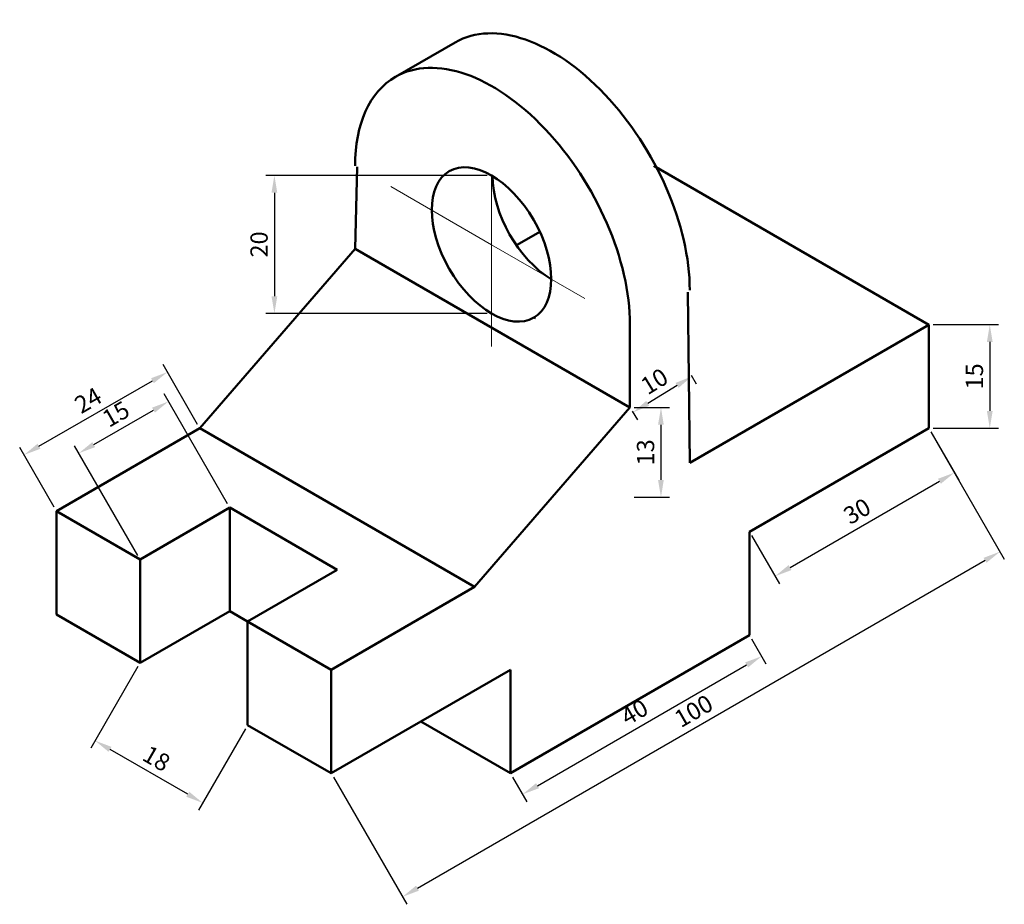
# Model space of a CAD drawing. Units: millimetres. Extents: x 20220 to 20363, y 7548 to 7676.
import ezdxf

# ---------------------------------------------------------------- set-up
doc = ezdxf.new("R2010")
doc.units = ezdxf.units.MM
doc.linetypes.add('CENTER', pattern=[50.8, 31.75, -6.35, 6.35, -6.35])
for name, color, linetype, lineweight in [('M-CNTR', 1, 'CENTER', 18), ('M-DIMS', 2, 'Continuous', 25), ('M-OUTL', 7, 'Continuous', 50)]:
    doc.layers.add(name, color=color, linetype=linetype, lineweight=lineweight)
doc.styles.get("Standard").update_dxf_attribs({"font": 'arial.ttf'})
doc.dimstyles.new('ISO-25', dxfattribs={"dimtxt": 2.5, "dimasz": 2.5, "dimexe": 1.25, "dimexo": 0.625, "dimtad": 1, "dimtxsty": 'Standard', "dimcen": 2.5, "dimadec": 0, "dimazin": 0, "dimtfac": 1, "dimtmove": 0, "dimatfit": 3, "dimfxl": 1, "dimarcsym": 0})

# ---------------------------------------------------------------- blocks, each defined once
blk = doc.blocks.new('*D1')
at = {"layer": 'Defpoints', "color": 0, "transparency": 16777216}
for p in [(20241.42, 7620.43), (20250.3, 7605.06), (20237.31, 7597.56)]:
    blk.add_point(p, dxfattribs=at)
at = {"layer": 'M-DIMS', "color": 0, "lineweight": -2, "transparency": 16777216}
for p, q in [((20249.98, 7605.6), (20240.79, 7621.52)), ((20230.59, 7614.18), (20239.25, 7619.18)), ((20236.99, 7598.1), (20227.8, 7614.02))]:
    blk.add_line(p, q, dxfattribs=at)
at = {"layer": 'M-DIMS', "color": 0, "transparency": 16777216}
for points in [[(20239.05, 7619.54), (20239.46, 7618.82), (20241.42, 7620.43)], [(20230.39, 7614.54), (20230.8, 7613.82), (20228.43, 7612.93)]]:
    blk.add_solid(points, dxfattribs=at)
at = {"layer": 'M-DIMS', "color": 0, "transparency": 16777216, "insert": (20233.97, 7618.33), "char_height": 2.5, "attachment_point": 5, "rotation": 30}
blk.add_mtext('15', dxfattribs=at)
blk = doc.blocks.new('*D2')
at = {"layer": 'Defpoints', "color": 0, "transparency": 16777216}
for p in [(20241.27, 7624.69), (20245.97, 7616.56), (20225.18, 7604.56)]:
    blk.add_point(p, dxfattribs=at)
at = {"layer": 'M-DIMS', "color": 0, "lineweight": -2, "transparency": 16777216}
for p, q in [((20245.65, 7617.1), (20240.65, 7625.77)), ((20222.65, 7613.94), (20239.11, 7623.44)), ((20224.87, 7605.1), (20219.86, 7613.77))]:
    blk.add_line(p, q, dxfattribs=at)
at = {"layer": 'M-DIMS', "color": 0, "transparency": 16777216}
for points in [[(20238.9, 7623.8), (20239.31, 7623.08), (20241.27, 7624.69)], [(20222.44, 7614.3), (20222.86, 7613.58), (20220.49, 7612.69)]]:
    blk.add_solid(points, dxfattribs=at)
at = {"layer": 'M-DIMS', "color": 0, "transparency": 16777216, "insert": (20229.94, 7620.32), "char_height": 2.5, "attachment_point": 5, "rotation": 30}
blk.add_mtext('24', dxfattribs=at)
blk = doc.blocks.new('*D3')
at = {"layer": 'Defpoints', "color": 0, "transparency": 16777216}
for p in [(20351.62, 7616.56), (20361.95, 7598.67), (20265.02, 7566.56)]:
    blk.add_point(p, dxfattribs=at)
at = {"layer": 'M-DIMS', "color": 0, "lineweight": -2, "transparency": 16777216}
for p, q in [((20351.93, 7616.02), (20362.58, 7597.58)), ((20277.51, 7549.92), (20359.79, 7597.42)), ((20265.33, 7566.02), (20275.97, 7547.58))]:
    blk.add_line(p, q, dxfattribs=at)
at = {"layer": 'M-DIMS', "color": 0, "transparency": 16777216}
for points in [[(20359.58, 7597.78), (20359.99, 7597.06), (20361.95, 7598.67)], [(20277.31, 7550.28), (20277.72, 7549.56), (20275.35, 7548.67)]]:
    blk.add_solid(points, dxfattribs=at)
at = {"layer": 'M-DIMS', "color": 0, "transparency": 16777216, "insert": (20317.7, 7575.31), "char_height": 2.5, "attachment_point": 5, "rotation": 30}
blk.add_mtext('100', dxfattribs=at)
blk = doc.blocks.new('*D4')
at = {"layer": 'Defpoints', "color": 0, "transparency": 16777216}
for p in [(20325.64, 7586.56), (20327.4, 7583.52), (20291, 7566.56)]:
    blk.add_point(p, dxfattribs=at)
at = {"layer": 'M-DIMS', "color": 0, "lineweight": -2, "transparency": 16777216}
for p, q in [((20325.95, 7586.02), (20328.02, 7582.43)), ((20294.92, 7564.77), (20325.23, 7582.27)), ((20291.31, 7566.02), (20293.38, 7562.43))]:
    blk.add_line(p, q, dxfattribs=at)
at = {"layer": 'M-DIMS', "color": 0, "transparency": 16777216}
for points in [[(20325.02, 7582.63), (20325.44, 7581.9), (20327.4, 7583.52)], [(20294.71, 7565.13), (20295.13, 7564.4), (20292.76, 7563.52)]]:
    blk.add_solid(points, dxfattribs=at)
at = {"layer": 'M-DIMS', "color": 0, "transparency": 16777216, "insert": (20309.13, 7575.16), "char_height": 2.5, "attachment_point": 5, "rotation": 30}
blk.add_mtext('40', dxfattribs=at)
blk = doc.blocks.new('*D5')
at = {"layer": 'Defpoints', "color": 0, "transparency": 16777216}
for p in [(20351.62, 7616.56), (20355.34, 7610.12), (20325.64, 7601.56)]:
    blk.add_point(p, dxfattribs=at)
at = {"layer": 'M-DIMS', "color": 0, "lineweight": -2, "transparency": 16777216}
for p, q in [((20351.93, 7616.02), (20355.97, 7609.03)), ((20331.52, 7596.37), (20353.18, 7608.87)), ((20325.95, 7601.02), (20329.98, 7594.03))]:
    blk.add_line(p, q, dxfattribs=at)
at = {"layer": 'M-DIMS', "color": 0, "transparency": 16777216}
for points in [[(20352.97, 7609.23), (20353.38, 7608.51), (20355.34, 7610.12)], [(20331.32, 7596.73), (20331.73, 7596.01), (20329.36, 7595.12)]]:
    blk.add_solid(points, dxfattribs=at)
at = {"layer": 'M-DIMS', "color": 0, "transparency": 16777216, "insert": (20341.4, 7604.26), "char_height": 2.5, "attachment_point": 5, "rotation": 30}
blk.add_mtext('30', dxfattribs=at)
blk = doc.blocks.new('*D6')
at = {"layer": 'Defpoints', "color": 0, "transparency": 16777216}
for p in [(20351.62, 7631.56), (20351.62, 7616.56), (20360.47, 7616.56)]:
    blk.add_point(p, dxfattribs=at)
at = {"layer": 'M-DIMS', "color": 0, "lineweight": -2, "transparency": 16777216}
for p, q in [((20352.25, 7631.56), (20361.72, 7631.56)), ((20360.47, 7629.06), (20360.47, 7619.06)), ((20352.25, 7616.56), (20361.72, 7616.56))]:
    blk.add_line(p, q, dxfattribs=at)
at = {"layer": 'M-DIMS', "color": 0, "transparency": 16777216}
for points in [[(20360.05, 7629.06), (20360.89, 7629.06), (20360.47, 7631.56)], [(20360.05, 7619.06), (20360.89, 7619.06), (20360.47, 7616.56)]]:
    blk.add_solid(points, dxfattribs=at)
at = {"layer": 'M-DIMS', "color": 0, "transparency": 16777216, "insert": (20358.57, 7624.06), "char_height": 2.5, "attachment_point": 5, "rotation": 90}
blk.add_mtext('15', dxfattribs=at)
blk = doc.blocks.new('*D7')
at = {"layer": 'Defpoints', "color": 0, "transparency": 16777216}
for p in [(20237.31, 7582.56), (20252.89, 7573.56), (20230.8, 7571.28)]:
    blk.add_point(p, dxfattribs=at)
at = {"layer": 'M-DIMS', "color": 0, "lineweight": -2, "transparency": 16777216}
for p, q in [((20236.99, 7582.02), (20230.17, 7570.2)), ((20252.58, 7573.02), (20245.76, 7561.2)), ((20244.22, 7563.53), (20232.96, 7570.03))]:
    blk.add_line(p, q, dxfattribs=at)
at = {"layer": 'M-DIMS', "color": 0, "transparency": 16777216}
for points in [[(20233.17, 7570.39), (20232.75, 7569.67), (20230.8, 7571.28)], [(20244.43, 7563.89), (20244.01, 7563.17), (20246.38, 7562.28)]]:
    blk.add_solid(points, dxfattribs=at)
at = {"layer": 'M-DIMS', "color": 0, "transparency": 16777216, "insert": (20239.54, 7568.43), "char_height": 2.5, "attachment_point": 5, "rotation": 330}
blk.add_mtext('18', dxfattribs=at)
blk = doc.blocks.new('*D8')
at = {"layer": 'Defpoints', "color": 0, "transparency": 16777216}
for p in [(20308.32, 7619.56), (20308.32, 7606.56), (20312.81, 7606.56)]:
    blk.add_point(p, dxfattribs=at)
at = {"layer": 'M-DIMS', "color": 0, "lineweight": -2, "transparency": 16777216}
for p, q in [((20308.95, 7619.56), (20314.06, 7619.56)), ((20312.81, 7617.06), (20312.81, 7609.06)), ((20308.95, 7606.56), (20314.06, 7606.56))]:
    blk.add_line(p, q, dxfattribs=at)
at = {"layer": 'M-DIMS', "color": 0, "transparency": 16777216}
for points in [[(20312.39, 7617.06), (20313.22, 7617.06), (20312.81, 7619.56)], [(20312.39, 7609.06), (20313.22, 7609.06), (20312.81, 7606.56)]]:
    blk.add_solid(points, dxfattribs=at)
at = {"layer": 'M-DIMS', "color": 0, "transparency": 16777216, "insert": (20310.9, 7613.06), "char_height": 2.5, "attachment_point": 5, "rotation": 90}
blk.add_mtext('13', dxfattribs=at)
blk = doc.blocks.new('*D9')
at = {"layer": 'Defpoints', "color": 0, "transparency": 16777216}
for p in [(20316.85, 7624.78), (20308.32, 7619.56), (20308.75, 7618.85)]:
    blk.add_point(p, dxfattribs=at)
at = {"layer": 'M-DIMS', "color": 0, "lineweight": -2, "transparency": 16777216}
for p, q in [((20317.18, 7624.25), (20317.93, 7623.01)), ((20315.15, 7622.77), (20310.89, 7620.16)), ((20308.65, 7619.03), (20309.41, 7617.79))]:
    blk.add_line(p, q, dxfattribs=at)
at = {"layer": 'M-DIMS', "color": 0, "transparency": 16777216}
for points in [[(20314.93, 7623.12), (20315.37, 7622.41), (20317.28, 7624.07)], [(20310.67, 7620.51), (20311.1, 7619.8), (20308.75, 7618.85)]]:
    blk.add_solid(points, dxfattribs=at)
at = {"layer": 'M-DIMS', "color": 0, "transparency": 16777216, "insert": (20312.02, 7623.08), "char_height": 2.5, "attachment_point": 5, "rotation": 31.4807}
blk.add_mtext('10', dxfattribs=at)
blk = doc.blocks.new('*D10')
at = {"layer": 'Defpoints', "color": 0, "transparency": 16777216}
for p in [(20288.24, 7653.18), (20256.78, 7633.18), (20288.24, 7633.18)]:
    blk.add_point(p, dxfattribs=at)
at = {"layer": 'M-DIMS', "color": 0, "lineweight": -2, "transparency": 16777216}
for p, q in [((20287.62, 7653.18), (20255.53, 7653.18)), ((20256.78, 7650.68), (20256.78, 7635.68)), ((20287.62, 7633.18), (20255.53, 7633.18))]:
    blk.add_line(p, q, dxfattribs=at)
at = {"layer": 'M-DIMS', "color": 0, "transparency": 16777216}
for points in [[(20256.36, 7650.68), (20257.2, 7650.68), (20256.78, 7653.18)], [(20256.36, 7635.68), (20257.2, 7635.68), (20256.78, 7633.18)]]:
    blk.add_solid(points, dxfattribs=at)
at = {"layer": 'M-DIMS', "color": 0, "transparency": 16777216, "insert": (20254.88, 7643.18), "char_height": 2.5, "attachment_point": 5, "rotation": 90}
blk.add_mtext('20', dxfattribs=at)

msp = doc.modelspace()

# ---------------------------------------------------------------- linework, layer by layer
at = {"layer": 'M-CNTR'}
for p, q in [((20288.245, 7653.185), (20288.245, 7628.407)), ((20288.245, 7643.149), (20273.679, 7651.558)), ((20288.245, 7643.149), (20301.775, 7635.337))]:
    msp.add_line(p, q, dxfattribs=at)
at = {"layer": 'M-OUTL'}
for p, q in [((20282.978, 7672.453), (20274.317, 7667.453)), ((20268.483, 7642.558), (20268.788, 7654.414)), ((20351.622, 7631.558), (20311.785, 7654.558)), ((20291.866, 7643.058), (20295.33, 7645.058)), ((20268.483, 7642.558), (20245.967, 7616.558)), ((20308.32, 7619.558), (20268.483, 7642.558)), ((20316.981, 7611.558), (20316.723, 7636.28)), ((20308.32, 7631.558), (20308.32, 7619.558)), ((20351.622, 7631.558), (20316.981, 7611.558)), ((20351.622, 7616.558), (20351.622, 7631.558)), ((20308.32, 7619.558), (20308.32, 7626.97)), ((20308.32, 7619.558), (20285.804, 7593.558)), ((20245.967, 7616.558), (20225.182, 7604.558)), ((20285.804, 7593.558), (20245.967, 7616.558)), ((20325.641, 7601.558), (20351.622, 7616.558)), ((20225.182, 7604.558), (20237.306, 7597.558)), ((20225.182, 7604.558), (20225.182, 7589.558)), ((20237.306, 7597.558), (20250.297, 7605.058)), ((20250.297, 7605.058), (20265.885, 7596.058)), ((20250.297, 7605.058), (20250.297, 7590.058)), ((20325.641, 7586.558), (20325.641, 7601.558)), ((20237.306, 7582.558), (20237.306, 7597.558)), ((20265.885, 7596.058), (20252.895, 7588.558)), ((20265.019, 7581.558), (20285.804, 7593.558)), ((20237.306, 7582.558), (20250.297, 7590.058)), ((20250.297, 7590.058), (20252.895, 7588.558)), ((20225.182, 7589.558), (20237.306, 7582.558)), ((20252.895, 7588.558), (20265.019, 7581.558)), ((20252.895, 7588.558), (20252.895, 7573.558)), ((20291, 7566.558), (20325.641, 7586.558)), ((20325.641, 7586.558), (20291, 7566.558)), ((20291, 7581.558), (20265.019, 7566.558)), ((20291, 7581.558), (20265.019, 7566.558)), ((20265.019, 7566.558), (20265.019, 7581.558)), ((20291, 7566.558), (20291, 7581.558)), ((20291, 7566.558), (20278.01, 7574.058)), ((20252.895, 7573.558), (20265.019, 7566.558))]:
    msp.add_line(p, q, dxfattribs=at)
for centre, major_axis, start_param, end_param in [((20297.062, 7648.058), (14.085, -24.395), 0.7853982, 3.1415927), ((20288.402, 7643.058), (14.085, -24.395), 0.7853982, 3.1415927), ((20288.402, 7643.058), (14.085, -24.395), 3.1415927, 3.9269908), ((20297.062, 7648.058), (6.124, -10.607), 3.9235752, 5.479659), ((20296.87, 7640.837), (6.124, -10.607), 3.1540262, 3.1556833), ((20296.87, 7640.837), (6.124, -10.607), 5.2150462, 5.2326687)]:
    msp.add_ellipse(centre, major_axis=major_axis, ratio=0.5773503, start_param=start_param, end_param=end_param, dxfattribs=at)
msp.add_ellipse((20288.245, 7643.185), major_axis=(6.124, -10.607), ratio=0.5773503, dxfattribs=at)

# ---------------------------------------------------------------- dimensions: what is measured, and where the dimension line sits
at = {"layer": 'M-DIMS'}
for base, p1, p2, picture, middle in [((20256.781, 7633.185), (20288.245, 7653.185), (20288.245, 7633.185), '*D10', (20254.88, 7643.185)), ((20312.806, 7606.558), (20308.32, 7619.558), (20308.32, 7606.558), '*D8', (20310.904, 7613.058))]:
    dim = msp.add_linear_dim(base=base, p1=p1, p2=p2, angle=90, dimstyle='ISO-25', override={"dimclrd": 0, "dimclre": 0, "dimclrt": 0}, dxfattribs=at)
    dim.commit()
    dim.dimension.update_dxf_attribs({"geometry": picture, "text_midpoint": middle})
for p1, p2, distance, picture, middle in [((20351.622, 7631.558), (20351.622, 7616.558), 8.848, '*D6', (20358.569, 7624.058)), ((20225.182, 7604.558), (20245.967, 7616.558), 9.392, '*D2', (20229.938, 7620.32)), ((20316.849, 7624.78), (20308.32, 7619.558), 0.829, '*D9', (20312.024, 7623.084)), ((20237.306, 7597.558), (20250.297, 7605.058), 17.754, '*D1', (20233.974, 7618.33)), ((20265.019, 7566.558), (20351.622, 7616.558), -20.66, '*D3', (20317.7, 7575.313)), ((20325.641, 7601.558), (20351.622, 7616.558), -7.437, '*D5', (20341.399, 7604.265)), ((20291, 7566.558), (20325.641, 7586.558), -3.513, '*D4', (20309.126, 7575.162)), ((20252.895, 7573.558), (20237.306, 7582.558), 13.02, '*D7', (20239.541, 7568.429))]:
    dim = msp.add_aligned_dim(p1=p1, p2=p2, distance=distance, dimstyle='ISO-25', override={"dimclrd": 0, "dimclre": 0, "dimclrt": 0}, dxfattribs=at)
    dim.commit()
    dim.dimension.update_dxf_attribs({"geometry": picture, "text_midpoint": middle})

doc.saveas('drawing.dxf')
